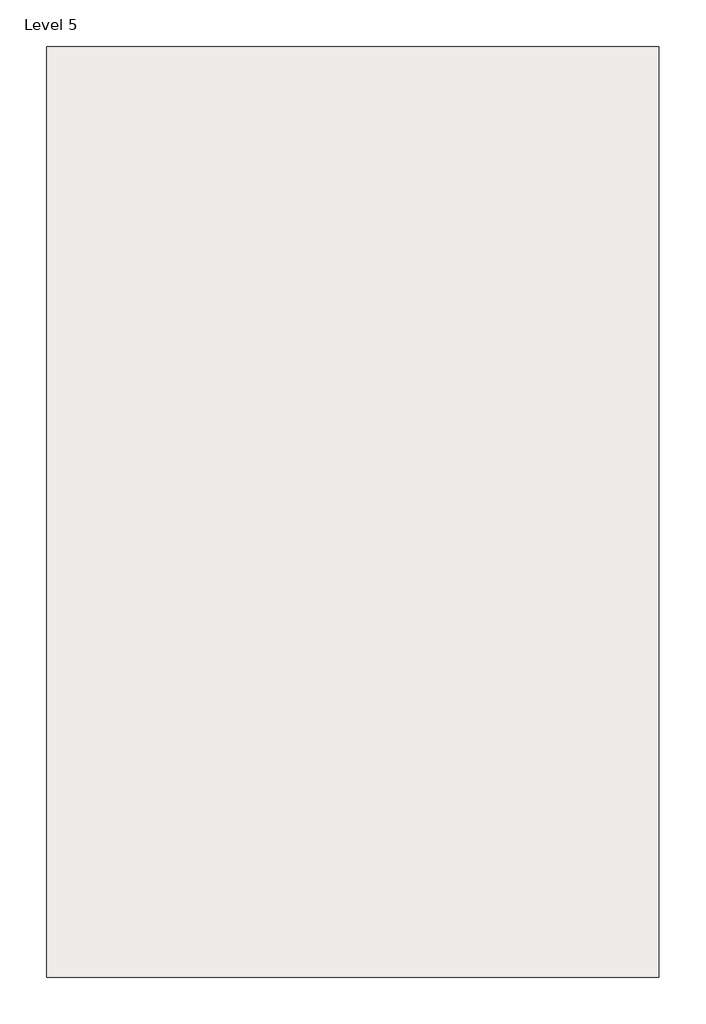
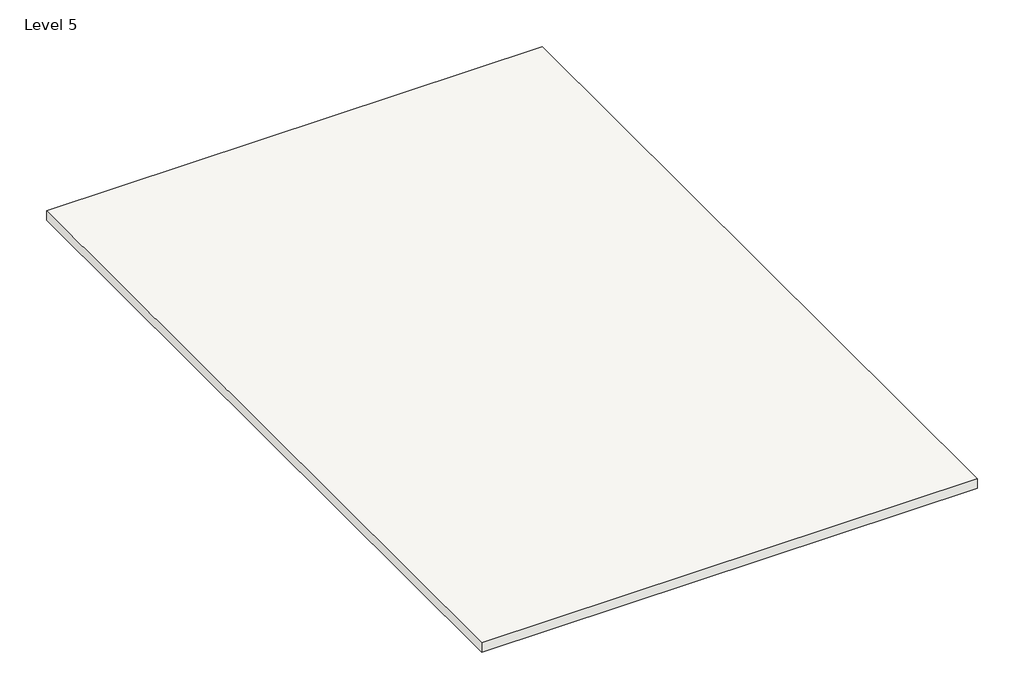
# One storey: 1 roof.
"""IFC4 building model written with IfcOpenShell, lengths in millimetres."""

from ifc_helpers import new_model, si_unit, frame, origin, place, context, project, spatial, polyline, outline, extrude, element, save

model = new_model("IFC4")

# Units and contexts
model_context = context("Model", 3, world=origin())
ifc_project = project(units=[si_unit("LENGTHUNIT", "METRE", prefix="MILLI")], contexts=[model_context])

# Site, building, storey
site = spatial("IfcSite", under=ifc_project)
building = spatial("IfcBuilding", under=site)
storey = spatial("IfcBuildingStorey", under=building, Name="Level 5", Elevation=12192.0)

# Roof
placement = place(None, origin())
element("IfcRoof", 1, ObjectType="Generic - 12\"", at=placement, inside=storey, context=model_context, shape_type="SweptSolid", body=[
    extrude(outline(polyline([(1524.0, 14055.3323212), (9144.0, 14055.3323212), (9144.0, 2472.9323212), (1524.0, 2472.9323212), (1524.0, 14055.3323212)])), frame((0.0, 0.0, 12192.0), z_axis=(0.0, 0.0, 1.0), x_axis=(1.0, 0.0, 0.0)), (0.0, 0.0, 1.0), 152.4),
])

save(model, "model.ifc")

# Revit data of these elements
# Type "Generic - 12\""
#   Assembly Code = "B1020"
#   Layers, outside or top first: 0' - 6" no material (function 1)
# Element 1 (IfcRoof, "Generic - 12\"")
#   built-in parameter 1001705 = 40.5 (stored number, unit not read)
#   built-in parameter 1001710 = 33615
#   Phase Created = New Construction
#   Materials on its faces: "Clad - White", "Default Roof", "Carpet (1)"
# Materials
#   "Clad - White": class "Wood", colour RGB 242 242 238, transparency 0, Cost = 0
#   "Default Roof": colour RGB 88 101 114, transparency 0, Cost = 0
#   "Carpet (1)": class "Carpet", colour RGB 124 80 67, transparency 0, Description = "Interior finish", Cost = 0
